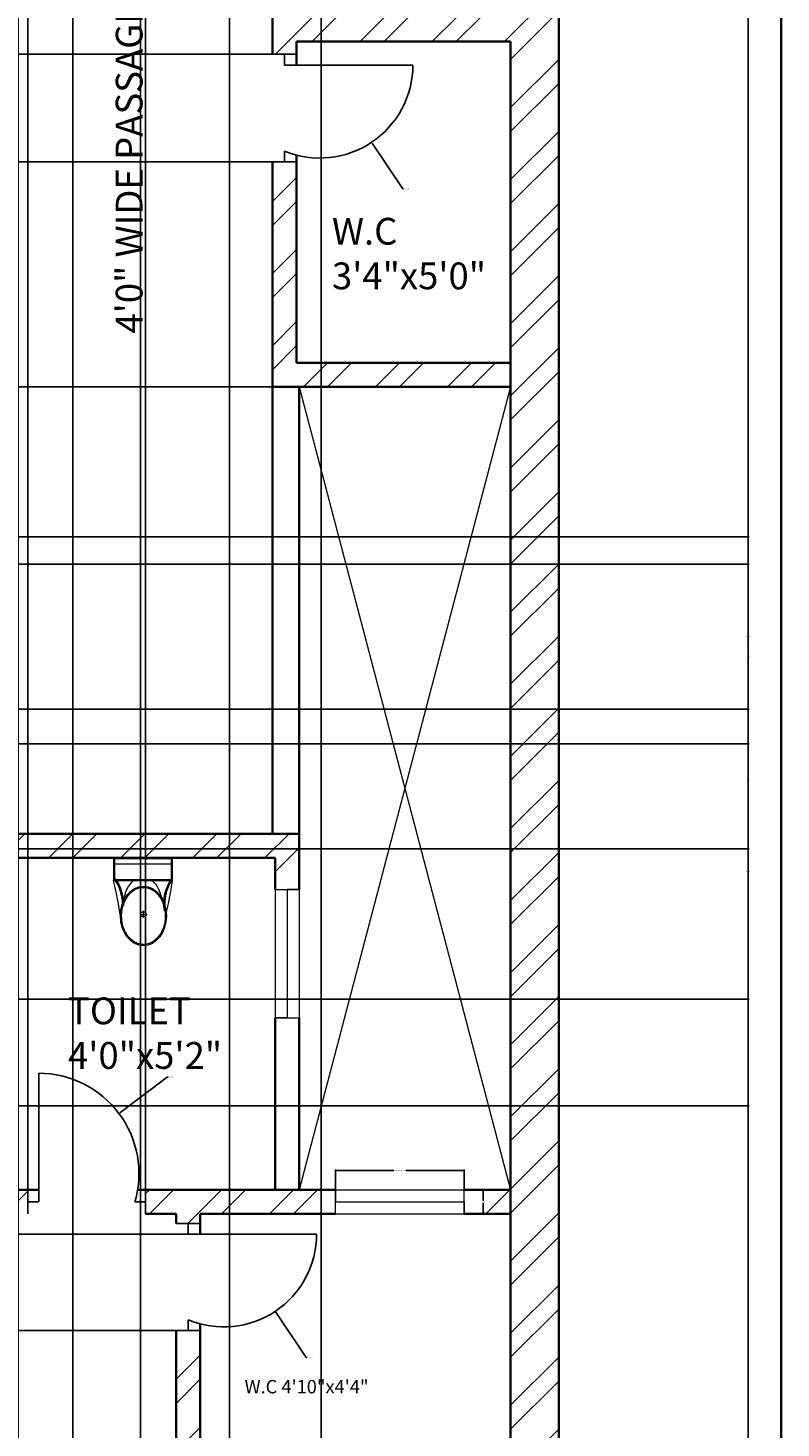
# Model space of a CAD drawing. Units: inches. Extents: x 2529 to 3014, y 1203 to 2262.
# Tile 9 of 13: x 2873 to 3014, y 1746 to 2008. Entities that reach past the tile are written whole.
import ezdxf

# ---------------------------------------------------------------- set-up
doc = ezdxf.new("R2010")
doc.units = ezdxf.units.IN
for name, color, linetype, lineweight in [('A-ANNO-DIMS', 2, 'Continuous', 18), ('A-ANNO-TTLB', 7, 'Continuous', 35), ('A-AREA-IDEN', 7, 'Continuous', 18), ('A-DOOR', 21, 'Continuous', 25), ('A-FLOR-FIXT', 8, 'Continuous', 18), ('A-FLOR-OPEN', 61, 'Continuous', 13), ('A-GLAZ', 191, 'Continuous', 18), ('A-WALL', 7, 'Continuous', 35), ('A-WALL-PATT', 143, 'Continuous', 13)]:
    doc.layers.add(name, color=color, linetype=linetype, lineweight=lineweight)
doc.styles.get("Standard").update_dxf_attribs({"font": 'arial.ttf'})
doc.dimstyles.get("Standard").update_dxf_attribs({"dimtxt": 0.18, "dimasz": 0.18, "dimexe": 0.18, "dimexo": 0.0625, "dimgap": 0.09, "dimtad": 0, "dimtih": 1, "dimtoh": 1, "dimdec": 4, "dimzin": 0, "dimdsep": 46, "dimtxsty": 'Standard', "dimcen": 0.09, "dimadec": 0, "dimazin": 0, "dimtfac": 1, "dimtdec": 4, "dimtofl": 0, "dimtmove": 0, "dimatfit": 3, "dimfxl": 1, "dimtolj": 1, "dimtzin": 0, "dimarcsym": 0})

# ---------------------------------------------------------------- blocks, each defined once
blk = doc.blocks.new('A$C31115884')
for p, q in [((283, 498), (223, 498)), ((258, 466), (258, 523)), ((0, 200), (0, 0)), ((520, 200), (0, 200)), ((10, 190), (10, 10)), ((510, 190), (10, 190)), ((510, 10), (510, 190)), ((520, 0), (520, 200)), ((510, 54), (0, 54)), ((10, 10), (510, 10)), ((0, 0), (520, 0))]:
    blk.add_line(p, q)
blk.add_circle((256, 496), 23.6)
for centre, radius, start, end in [((2778, -205), 2807, 165.4549, 171.7133), ((3237, 905), 2807, 188.2867, 194.5451), ((-295, 403), 365, 324.2091, 9.3499), ((-295, 403), 375, 324.2091, 9.3499), ((139, 406), 293, 315.8436, 2.6563), ((806, 403), 375, 179.2036, 215.7909), ((806, 403), 365, 170.6501, 215.7909), ((384, 406), 293, 190.2774, 224.1564)]:
    blk.add_arc(centre, radius, start, end)
blk.add_ellipse((256, 510), major_axis=(0, -261), ratio=0.772727)
blk.add_open_spline([(256, 259), (263, 259), (270, 260), (288, 262), (299, 265), (320, 273), (330, 278), (350, 291), (360, 299), (378, 316), (386, 326), (402, 347), (409, 358), (421, 383), (427, 395), (436, 422), (440, 436), (445, 465), (447, 480), (448, 509), (448, 524), (445, 553), (443, 568), (436, 596), (432, 610), (422, 636), (416, 649), (402, 672), (395, 683), (379, 703), (370, 712), (351, 728), (341, 735), (321, 746), (310, 751), (289, 757), (278, 759), (256, 761), (245, 761), (223, 757), (212, 754), (191, 746), (181, 741), (161, 728), (151, 720), (133, 703), (125, 693), (110, 672), (103, 660), (90, 636), (85, 623), (76, 596), (72, 582), (67, 553), (66, 538), (64, 509), (65, 494), (68, 465), (70, 450), (77, 422), (81, 408), (91, 382), (97, 370), (111, 346), (118, 335), (135, 316), (144, 307), (162, 291), (172, 284), (193, 273), (203, 269), (225, 262), (236, 260), (250, 259), (253, 259), (256, 259)], degree=3, knots=[0, 0, 0, 0, 0.110105, 0.110105, 0.285049, 0.285049, 0.459994, 0.459994, 0.634938, 0.634938, 0.809882, 0.809882, 0.984827, 0.984827, 1.159771, 1.159771, 1.334715, 1.334715, 1.50966, 1.50966, 1.684604, 1.684604, 1.859549, 1.859549, 2.034493, 2.034493, 2.209437, 2.209437, 2.384382, 2.384382, 2.559326, 2.559326, 2.73427, 2.73427, 2.909215, 2.909215, 3.084159, 3.084159, 3.259103, 3.259103, 3.434048, 3.434048, 3.608992, 3.608992, 3.783936, 3.783936, 3.958881, 3.958881, 4.133825, 4.133825, 4.30877, 4.30877, 4.483714, 4.483714, 4.658658, 4.658658, 4.833603, 4.833603, 5.008547, 5.008547, 5.183491, 5.183491, 5.358436, 5.358436, 5.53338, 5.53338, 5.708324, 5.708324, 5.883269, 5.883269, 6.058213, 6.058213, 6.233158, 6.233158, 6.283185, 6.283185, 6.283185, 6.283185])
blk = doc.blocks.new('WIN-24x4-5')
for p, q in [((0, 24), (4.5, 24)), ((0, 24), (0, 0)), ((4.5, 24), (2.25, 24)), ((2.25, 24), (2.25, 0)), ((4.5, 24), (4.5, 0)), ((2.25, 0), (0, 0)), ((0, 0), (4.5, 0))]:
    blk.add_line(p, q)
blk = doc.blocks.new('*D12')
at = {"layer": 'A-ANNO-DIMS', "color": 0, "lineweight": -2, "transparency": 16777216}
for p, q in [((2930.37, 1791.07), (2930.37, 1794.78)), ((2930.55, 1794.6), (2941.25, 1794.6)), ((2954.19, 1794.6), (2943.49, 1794.6)), ((2954.37, 1791.07), (2954.37, 1794.78))]:
    blk.add_line(p, q, dxfattribs=at)
at = {"layer": 'A-ANNO-DIMS', "color": 0, "transparency": 16777216}
for points in [[(2930.55, 1794.63), (2930.55, 1794.57), (2930.37, 1794.6)], [(2954.19, 1794.63), (2954.19, 1794.57), (2954.37, 1794.6)]]:
    blk.add_solid(points, dxfattribs=at)
at = {"layer": 'Defpoints', "color": 0, "transparency": 16777216}
for p in [(2930.37, 1794.6), (2930.37, 1791), (2954.37, 1791)]:
    blk.add_point(p, dxfattribs=at)
at = {"layer": 'A-ANNO-DIMS', "color": 0, "transparency": 16777216, "insert": (2942.37, 1794.6), "char_height": 0.18, "attachment_point": 5}
blk.add_mtext('\\A1;WINDOW 24 TYP.', dxfattribs=at)
blk = doc.blocks.new('*D13')
at = {"layer": 'A-ANNO-DIMS', "color": 0, "lineweight": -2, "transparency": 16777216}
for p, q in [((2954.43, 1791), (2958.15, 1791)), ((2957.97, 1790.82), (2957.97, 1788.93)), ((2957.97, 1786.68), (2957.97, 1788.57)), ((2954.43, 1786.5), (2958.15, 1786.5))]:
    blk.add_line(p, q, dxfattribs=at)
at = {"layer": 'A-ANNO-DIMS', "color": 0, "transparency": 16777216}
for points in [[(2957.94, 1790.82), (2958, 1790.82), (2957.97, 1791)], [(2957.94, 1786.68), (2958, 1786.68), (2957.97, 1786.5)]]:
    blk.add_solid(points, dxfattribs=at)
at = {"layer": 'Defpoints', "color": 0, "transparency": 16777216}
for p in [(2954.37, 1791), (2957.97, 1791), (2954.37, 1786.5)]:
    blk.add_point(p, dxfattribs=at)
at = {"layer": 'A-ANNO-DIMS', "color": 0, "transparency": 16777216, "insert": (2957.97, 1788.75), "char_height": 0.18, "attachment_point": 5}
blk.add_mtext('\\A1;5 TYP.', dxfattribs=at)
blk = doc.blocks.new('*D17')
at = {"layer": 'A-ANNO-DIMS', "color": 0, "lineweight": -2, "transparency": 16777216}
for p, q in [((2972.12, 2207.5), (3007.66, 2207.5)), ((3007.48, 2207.32), (3007.48, 1890.69)), ((3007.48, 1573.68), (3007.48, 1890.32)), ((2972.12, 1573.5), (3007.66, 1573.5))]:
    blk.add_line(p, q, dxfattribs=at)
at = {"layer": 'A-ANNO-DIMS', "color": 0, "transparency": 16777216}
for points in [[(3007.45, 2207.32), (3007.51, 2207.32), (3007.48, 2207.5)], [(3007.45, 1573.68), (3007.51, 1573.68), (3007.48, 1573.5)]]:
    blk.add_solid(points, dxfattribs=at)
at = {"layer": 'Defpoints', "color": 0, "transparency": 16777216}
for p in [(2972.06, 2207.5), (3007.48, 2207.5), (2972.06, 1573.5)]:
    blk.add_point(p, dxfattribs=at)
at = {"layer": 'A-ANNO-DIMS', "color": 0, "transparency": 16777216, "insert": (3007.48, 1890.5), "char_height": 0.18, "attachment_point": 5}
blk.add_mtext('\\A1;634', dxfattribs=at)
blk = doc.blocks.new('*D39')
at = {"layer": 'A-ANNO-DIMS', "color": 0, "lineweight": -2, "transparency": 16777216}
for p, q in [((2848.27, 1734.07), (2848.27, 2243.11)), ((2848.45, 2242.93), (2864.3, 2242.93)), ((2881.08, 2242.93), (2865.23, 2242.93)), ((2881.26, 1734.07), (2881.26, 2243.11))]:
    blk.add_line(p, q, dxfattribs=at)
at = {"layer": 'A-ANNO-DIMS', "color": 0, "transparency": 16777216}
for points in [[(2848.45, 2242.96), (2848.45, 2242.9), (2848.27, 2242.93)], [(2881.08, 2242.96), (2881.08, 2242.9), (2881.26, 2242.93)]]:
    blk.add_solid(points, dxfattribs=at)
at = {"layer": 'Defpoints', "color": 0, "transparency": 16777216}
for p in [(2881.26, 2242.93), (2848.27, 1734), (2881.26, 1734)]:
    blk.add_point(p, dxfattribs=at)
at = {"layer": 'A-ANNO-DIMS', "color": 0, "transparency": 16777216, "insert": (2864.76, 2242.93), "char_height": 0.18, "attachment_point": 5}
blk.add_mtext('\\A1;32.994', dxfattribs=at)
blk = doc.blocks.new('*D57')
at = {"layer": 'A-ANNO-DIMS', "color": 0, "lineweight": -2, "transparency": 16777216}
for p, q in [((2871.06, 2198.44), (2871.06, 1483.77)), ((2893.92, 2198.44), (2893.92, 1483.77)), ((2871.24, 1483.95), (2882.02, 1483.95)), ((2893.74, 1483.95), (2882.95, 1483.95))]:
    blk.add_line(p, q, dxfattribs=at)
at = {"layer": 'A-ANNO-DIMS', "color": 0, "transparency": 16777216}
for points in [[(2871.24, 1483.98), (2871.24, 1483.92), (2871.06, 1483.95)], [(2893.74, 1483.98), (2893.74, 1483.92), (2893.92, 1483.95)]]:
    blk.add_solid(points, dxfattribs=at)
at = {"layer": 'Defpoints', "color": 0, "transparency": 16777216}
for p in [(2871.06, 2198.5), (2893.92, 2198.5), (2893.92, 1483.95)]:
    blk.add_point(p, dxfattribs=at)
at = {"layer": 'A-ANNO-DIMS', "color": 0, "transparency": 16777216, "insert": (2882.49, 1483.95), "char_height": 0.18, "attachment_point": 5}
blk.add_mtext('\\A1;22.866', dxfattribs=at)
blk = doc.blocks.new('*D60')
at = {"layer": 'A-ANNO-DIMS', "color": 0, "lineweight": -2, "transparency": 16777216}
for p, q in [((2918.49, 2003.13), (2541.45, 2003.13)), ((2541.63, 2002.95), (2541.63, 1993.28)), ((2541.63, 1983.24), (2541.63, 1992.91)), ((2918.49, 1983.06), (2541.45, 1983.06))]:
    blk.add_line(p, q, dxfattribs=at)
at = {"layer": 'A-ANNO-DIMS', "color": 0, "transparency": 16777216}
for points in [[(2541.6, 2002.95), (2541.66, 2002.95), (2541.63, 2003.13)], [(2541.6, 1983.24), (2541.66, 1983.24), (2541.63, 1983.06)]]:
    blk.add_solid(points, dxfattribs=at)
at = {"layer": 'Defpoints', "color": 0, "transparency": 16777216}
for p in [(2918.56, 2003.13), (2541.63, 1983.06), (2918.56, 1983.06)]:
    blk.add_point(p, dxfattribs=at)
at = {"layer": 'A-ANNO-DIMS', "color": 0, "transparency": 16777216, "insert": (2541.63, 1993.1), "char_height": 0.18, "attachment_point": 5}
blk.add_mtext('\\A1;20.077', dxfattribs=at)
blk = doc.blocks.new('*D61')
at = {"layer": 'A-ANNO-DIMS', "color": 0, "lineweight": -2, "transparency": 16777216}
for p, q in [((2918.49, 1983.06), (2541.45, 1983.06)), ((2541.63, 1982.88), (2541.63, 1962.21)), ((2541.63, 1941.18), (2541.63, 1961.85)), ((2918.49, 1941), (2541.45, 1941))]:
    blk.add_line(p, q, dxfattribs=at)
at = {"layer": 'A-ANNO-DIMS', "color": 0, "transparency": 16777216}
for points in [[(2541.6, 1982.88), (2541.66, 1982.88), (2541.63, 1983.06)], [(2541.6, 1941.18), (2541.66, 1941.18), (2541.63, 1941)]]:
    blk.add_solid(points, dxfattribs=at)
at = {"layer": 'Defpoints', "color": 0, "transparency": 16777216}
for p in [(2918.56, 1983.06), (2541.63, 1941), (2918.56, 1941)]:
    blk.add_point(p, dxfattribs=at)
at = {"layer": 'A-ANNO-DIMS', "color": 0, "transparency": 16777216, "insert": (2541.63, 1962.03), "char_height": 0.18, "attachment_point": 5}
blk.add_mtext('\\A1;42.05', dxfattribs=at)
blk = doc.blocks.new('*D62')
at = {"layer": 'A-ANNO-DIMS', "color": 0, "lineweight": -2, "transparency": 16777216}
for p, q in [((2904.99, 1782.69), (2541.45, 1782.69)), ((2541.63, 1782.51), (2541.63, 1773.88)), ((2541.63, 1764.89), (2541.63, 1773.52)), ((2904.99, 1764.71), (2541.45, 1764.71))]:
    blk.add_line(p, q, dxfattribs=at)
at = {"layer": 'A-ANNO-DIMS', "color": 0, "transparency": 16777216}
for points in [[(2541.6, 1782.51), (2541.66, 1782.51), (2541.63, 1782.69)], [(2541.6, 1764.89), (2541.66, 1764.89), (2541.63, 1764.71)]]:
    blk.add_solid(points, dxfattribs=at)
at = {"layer": 'Defpoints', "color": 0, "transparency": 16777216}
for p in [(2905.06, 1782.69), (2541.63, 1764.71), (2905.06, 1764.71)]:
    blk.add_point(p, dxfattribs=at)
at = {"layer": 'A-ANNO-DIMS', "color": 0, "transparency": 16777216, "insert": (2541.63, 1773.7), "char_height": 0.18, "attachment_point": 5}
blk.add_mtext('\\A1;17.983', dxfattribs=at)
blk = doc.blocks.new('*D63')
at = {"layer": 'A-ANNO-DIMS', "color": 0, "lineweight": -2, "transparency": 16777216}
for p, q in [((2737.62, 1907.87), (3007.66, 1907.87)), ((3007.48, 1907.69), (3007.48, 1894.52)), ((3007.48, 1880.99), (3007.48, 1894.16)), ((2737.62, 1880.81), (3007.66, 1880.81))]:
    blk.add_line(p, q, dxfattribs=at)
at = {"layer": 'A-ANNO-DIMS', "color": 0, "transparency": 16777216}
for points in [[(3007.45, 1907.69), (3007.51, 1907.69), (3007.48, 1907.87)], [(3007.45, 1880.99), (3007.51, 1880.99), (3007.48, 1880.81)]]:
    blk.add_solid(points, dxfattribs=at)
at = {"layer": 'Defpoints', "color": 0, "transparency": 16777216}
for p in [(2737.56, 1907.87), (3007.48, 1907.87), (2737.56, 1880.81)]:
    blk.add_point(p, dxfattribs=at)
at = {"layer": 'A-ANNO-DIMS', "color": 0, "transparency": 16777216, "insert": (3007.48, 1894.34), "char_height": 0.18, "attachment_point": 5}
blk.add_mtext('\\A1;27.057', dxfattribs=at)
blk = doc.blocks.new('*D64')
at = {"layer": 'A-ANNO-DIMS', "color": 0, "lineweight": -2, "transparency": 16777216}
for p, q in [((2872.87, 1791.07), (2872.87, 2243.11)), ((2873.05, 2242.93), (2883.47, 2242.93)), ((2894.68, 2242.93), (2884.26, 2242.93)), ((2894.86, 1791.07), (2894.86, 2243.11))]:
    blk.add_line(p, q, dxfattribs=at)
at = {"layer": 'A-ANNO-DIMS', "color": 0, "transparency": 16777216}
for points in [[(2873.05, 2242.96), (2873.05, 2242.9), (2872.87, 2242.93)], [(2894.68, 2242.96), (2894.68, 2242.9), (2894.86, 2242.93)]]:
    blk.add_solid(points, dxfattribs=at)
at = {"layer": 'Defpoints', "color": 0, "transparency": 16777216}
for p in [(2894.86, 2242.93), (2872.87, 1791), (2894.86, 1791)]:
    blk.add_point(p, dxfattribs=at)
at = {"layer": 'A-ANNO-DIMS', "color": 0, "transparency": 16777216, "insert": (2883.87, 2242.93), "char_height": 0.18, "attachment_point": 5}
blk.add_mtext('\\A1;21.99', dxfattribs=at)
blk = doc.blocks.new('*D67')
at = {"layer": 'A-ANNO-DIMS', "color": 0, "lineweight": -2, "transparency": 16777216}
for p, q in [((2678.12, 1913), (3007.66, 1913)), ((3007.48, 1912.82), (3007.48, 1893.83)), ((3007.48, 1874.48), (3007.48, 1893.47)), ((2678.12, 1874.3), (3007.66, 1874.3))]:
    blk.add_line(p, q, dxfattribs=at)
at = {"layer": 'A-ANNO-DIMS', "color": 0, "transparency": 16777216}
for points in [[(3007.45, 1912.82), (3007.51, 1912.82), (3007.48, 1913)], [(3007.45, 1874.48), (3007.51, 1874.48), (3007.48, 1874.3)]]:
    blk.add_solid(points, dxfattribs=at)
at = {"layer": 'Defpoints', "color": 0, "transparency": 16777216}
for p in [(2678.06, 1913), (3007.48, 1913), (2678.06, 1874.3)]:
    blk.add_point(p, dxfattribs=at)
at = {"layer": 'A-ANNO-DIMS', "color": 0, "transparency": 16777216, "insert": (3007.48, 1893.65), "char_height": 0.18, "attachment_point": 5}
blk.add_mtext('\\A1;38.7', dxfattribs=at)
blk = doc.blocks.new('*D68')
at = {"layer": 'A-ANNO-DIMS', "color": 0, "lineweight": -2, "transparency": 16777216}
for p, q in [((2622.12, 1874.3), (3007.66, 1874.3)), ((3007.48, 1874.12), (3007.48, 1850.62)), ((3007.48, 1826.75), (3007.48, 1850.25)), ((2622.12, 1826.57), (3007.66, 1826.57))]:
    blk.add_line(p, q, dxfattribs=at)
at = {"layer": 'A-ANNO-DIMS', "color": 0, "transparency": 16777216}
for points in [[(3007.45, 1874.12), (3007.51, 1874.12), (3007.48, 1874.3)], [(3007.45, 1826.75), (3007.51, 1826.75), (3007.48, 1826.57)]]:
    blk.add_solid(points, dxfattribs=at)
at = {"layer": 'Defpoints', "color": 0, "transparency": 16777216}
for p in [(2622.06, 1874.3), (3007.48, 1874.3), (2622.06, 1826.57)]:
    blk.add_point(p, dxfattribs=at)
at = {"layer": 'A-ANNO-DIMS', "color": 0, "transparency": 16777216, "insert": (3007.48, 1850.43), "char_height": 0.18, "attachment_point": 5}
blk.add_mtext('\\A1;47.735', dxfattribs=at)
blk = doc.blocks.new('*D69')
at = {"layer": 'A-ANNO-DIMS', "color": 0, "lineweight": -2, "transparency": 16777216}
for p, q in [((2737.62, 1854.67), (3007.66, 1854.67)), ((3007.48, 1854.49), (3007.48, 1830.85)), ((3007.48, 1806.85), (3007.48, 1830.49)), ((2737.62, 1806.67), (3007.66, 1806.67))]:
    blk.add_line(p, q, dxfattribs=at)
at = {"layer": 'A-ANNO-DIMS', "color": 0, "transparency": 16777216}
for points in [[(3007.45, 1854.49), (3007.51, 1854.49), (3007.48, 1854.67)], [(3007.45, 1806.85), (3007.51, 1806.85), (3007.48, 1806.67)]]:
    blk.add_solid(points, dxfattribs=at)
at = {"layer": 'Defpoints', "color": 0, "transparency": 16777216}
for p in [(2737.56, 1854.67), (3007.48, 1854.67), (2737.56, 1806.67)]:
    blk.add_point(p, dxfattribs=at)
at = {"layer": 'A-ANNO-DIMS', "color": 0, "transparency": 16777216, "insert": (3007.48, 1830.67), "char_height": 0.18, "attachment_point": 5}
blk.add_mtext('\\A1;48', dxfattribs=at)
blk = doc.blocks.new('*D70')
at = {"layer": 'A-ANNO-DIMS', "color": 0, "lineweight": -2, "transparency": 16777216}
for p, q in [((2737.62, 1880.81), (3007.66, 1880.81)), ((3007.48, 1880.63), (3007.48, 1867.92)), ((3007.48, 1854.85), (3007.48, 1867.56)), ((2737.62, 1854.67), (3007.66, 1854.67))]:
    blk.add_line(p, q, dxfattribs=at)
at = {"layer": 'A-ANNO-DIMS', "color": 0, "transparency": 16777216}
for points in [[(3007.45, 1880.63), (3007.51, 1880.63), (3007.48, 1880.81)], [(3007.45, 1854.85), (3007.51, 1854.85), (3007.48, 1854.67)]]:
    blk.add_solid(points, dxfattribs=at)
at = {"layer": 'Defpoints', "color": 0, "transparency": 16777216}
for p in [(2737.56, 1880.81), (3007.48, 1880.81), (2737.56, 1854.67)]:
    blk.add_point(p, dxfattribs=at)
at = {"layer": 'A-ANNO-DIMS', "color": 0, "transparency": 16777216, "insert": (3007.48, 1867.74), "char_height": 0.18, "attachment_point": 5}
blk.add_mtext('\\A1;26.14', dxfattribs=at)
blk = doc.blocks.new('*D75')
at = {"layer": 'A-ANNO-DIMS', "color": 0, "lineweight": -2, "transparency": 16777216}
for p, q in [((2893.92, 2187.06), (2893.92, 1483.77)), ((2910.52, 2189.17), (2910.52, 1483.77)), ((2894.1, 1483.95), (2901.91, 1483.95)), ((2910.34, 1483.95), (2902.54, 1483.95))]:
    blk.add_line(p, q, dxfattribs=at)
at = {"layer": 'A-ANNO-DIMS', "color": 0, "transparency": 16777216}
for points in [[(2894.1, 1483.98), (2894.1, 1483.92), (2893.92, 1483.95)], [(2910.34, 1483.98), (2910.34, 1483.92), (2910.52, 1483.95)]]:
    blk.add_solid(points, dxfattribs=at)
at = {"layer": 'Defpoints', "color": 0, "transparency": 16777216}
for p in [(2893.92, 2187.12), (2910.52, 2189.24), (2910.52, 1483.95)]:
    blk.add_point(p, dxfattribs=at)
at = {"layer": 'A-ANNO-DIMS', "color": 0, "transparency": 16777216, "insert": (2902.22, 1483.95), "char_height": 0.18, "attachment_point": 5}
blk.add_mtext('\\A1;16.6', dxfattribs=at)
blk = doc.blocks.new('*D76')
at = {"layer": 'A-ANNO-DIMS', "color": 0, "lineweight": -2, "transparency": 16777216}
for p, q in [((2910.52, 2189.17), (2910.52, 1483.77)), ((2927.64, 2189.17), (2927.64, 1483.77)), ((2910.7, 1483.95), (2918.63, 1483.95)), ((2927.46, 1483.95), (2919.54, 1483.95))]:
    blk.add_line(p, q, dxfattribs=at)
at = {"layer": 'A-ANNO-DIMS', "color": 0, "transparency": 16777216}
for points in [[(2910.7, 1483.98), (2910.7, 1483.92), (2910.52, 1483.95)], [(2927.46, 1483.98), (2927.46, 1483.92), (2927.64, 1483.95)]]:
    blk.add_solid(points, dxfattribs=at)
at = {"layer": 'Defpoints', "color": 0, "transparency": 16777216}
for p in [(2910.52, 2189.24), (2927.64, 2189.24), (2927.64, 1483.95)]:
    blk.add_point(p, dxfattribs=at)
at = {"layer": 'A-ANNO-DIMS', "color": 0, "transparency": 16777216, "insert": (2919.08, 1483.95), "char_height": 0.18, "attachment_point": 5}
blk.add_mtext('\\A1;17.123', dxfattribs=at)
blk = doc.blocks.new('*D88')
at = {"layer": 'A-ANNO-DIMS', "color": 0, "lineweight": -2, "transparency": 16777216}
for p, q in [((2898.87, 1812), (2890.02, 1805.36)), ((2899.05, 1812), (2898.87, 1812)), ((2874.78, 1794.01), (2874.96, 1794.01)), ((2874.87, 1793.92), (2874.87, 1794.1))]:
    blk.add_line(p, q, dxfattribs=at)
at = {"layer": 'A-ANNO-DIMS', "color": 0, "transparency": 16777216}
blk.add_solid([(2890, 1805.38), (2890.03, 1805.34), (2889.87, 1805.25)], dxfattribs=at)
at = {"layer": 'Defpoints', "color": 0, "transparency": 16777216}
for p in [(2889.87, 1805.25), (2874.87, 1794.01)]:
    blk.add_point(p, dxfattribs=at)
at = {"layer": 'A-ANNO-DIMS', "color": 0, "transparency": 16777216, "insert": (2899.6, 1812), "char_height": 0.18, "attachment_point": 5}
blk.add_mtext('\\A1;R18.742', dxfattribs=at)
blk = doc.blocks.new('*D90')
at = {"layer": 'A-ANNO-DIMS', "color": 0, "lineweight": -2, "transparency": 16777216}
for p, q in [((2927.33, 2001.13), (2927.51, 2001.13)), ((2927.42, 2001.04), (2927.42, 2001.22)), ((2942.9, 1978.02), (2937.2, 1986.54)), ((2943.08, 1978.02), (2942.9, 1978.02))]:
    blk.add_line(p, q, dxfattribs=at)
at = {"layer": 'A-ANNO-DIMS', "color": 0, "transparency": 16777216}
blk.add_solid([(2937.22, 1986.56), (2937.17, 1986.52), (2937.1, 1986.69)], dxfattribs=at)
at = {"layer": 'Defpoints', "color": 0, "transparency": 16777216}
for p in [(2927.42, 2001.13), (2937.1, 1986.69)]:
    blk.add_point(p, dxfattribs=at)
at = {"layer": 'A-ANNO-DIMS', "color": 0, "transparency": 16777216, "insert": (2943.63, 1978.02), "char_height": 0.18, "attachment_point": 5}
blk.add_mtext('\\A1;R17.385', dxfattribs=at)
blk = doc.blocks.new('*D91')
at = {"layer": 'A-ANNO-DIMS', "color": 0, "lineweight": -2, "transparency": 16777216}
for p, q in [((2909.39, 1782.69), (2909.57, 1782.69)), ((2909.48, 1782.6), (2909.48, 1782.78)), ((2924.85, 1759.62), (2919.18, 1768.13)), ((2925.03, 1759.62), (2924.85, 1759.62))]:
    blk.add_line(p, q, dxfattribs=at)
at = {"layer": 'A-ANNO-DIMS', "color": 0, "transparency": 16777216}
blk.add_solid([(2919.21, 1768.14), (2919.16, 1768.11), (2919.08, 1768.28)], dxfattribs=at)
at = {"layer": 'Defpoints', "color": 0, "transparency": 16777216}
for p in [(2909.48, 1782.69), (2919.08, 1768.28)]:
    blk.add_point(p, dxfattribs=at)
at = {"layer": 'A-ANNO-DIMS', "color": 0, "transparency": 16777216, "insert": (2925.57, 1759.62), "char_height": 0.18, "attachment_point": 5}
blk.add_mtext('\\A1;R17.322', dxfattribs=at)

msp = doc.modelspace()

# ---------------------------------------------------------------- hatches: boundary and pattern name
at = {"layer": 'A-WALL-PATT'}
h = msp.add_hatch(dxfattribs=at)
h.set_pattern_fill('ANSI32', color=256)
h.paths.add_polyline_path([(2686.5554, 2106.5032), (2622.0554, 2106.5032), (2622.0554, 2109.2964), (2617.4223, 2109.2964), (2613.0554, 2109.2964), (2613.0554, 2106.5032), (2577.0554, 2106.5032), (2577.0554, 2092.6918), (2586.0554, 2092.6918), (2586.0554, 2102.0032), (2682.0554, 2102.0032), (2682.0554, 2099.9833), (2686.5554, 2099.9833), (2686.5554, 2102.0032)])
h.paths.add_polyline_path([(2695.2249, 2054.0032), (2686.5554, 2054.0032), (2686.5554, 2080.2316), (2684.3054, 2080.2316), (2682.0554, 2080.2316), (2682.0554, 2054.0032), (2586.0554, 2054.0032), (2586.0554, 2068.6918), (2577.0554, 2068.6918), (2577.0554, 2019.1229), (2586.0554, 2019.1229), (2586.0554, 2049.5032), (2695.2249, 2049.5032)])
h.paths.add_polyline_path([(2737.5554, 2049.5032), (2866.5554, 2049.5032), (2866.5554, 2045.0233), (2871.0554, 2045.0233), (2871.0554, 2049.5032), (2871.0554, 2172.5032), (2866.5554, 2172.5032), (2829.1265, 2172.5032), (2829.1265, 2168.0032), (2866.5554, 2168.0032), (2866.5554, 2054.0032), (2737.5554, 2054.0032), (2737.5554, 2056.4892), (2735.3054, 2056.4892), (2733.0554, 2056.4892), (2733.0554, 2049.5032), (2733.0554, 1917.5032), (2733.0554, 1913.0032), (2871.0554, 1913.0032), (2871.0554, 1924.9149), (2868.8054, 1924.9149), (2866.5554, 1924.9149), (2866.5554, 1917.5032), (2737.5554, 1917.5032)], flags=17)
h.paths.add_polyline_path([(2972.0554, 2207.5032), (2613.0554, 2207.5032), (2613.0554, 2205.5032), (2613.0554, 2188.9366), (2622.0554, 2188.9366), (2622.0554, 2198.5032), (2733.0554, 2198.5032), (2733.0554, 2084.8053), (2735.3054, 2084.8053), (2737.5554, 2084.8053), (2737.5554, 2168.0032), (2769.1265, 2168.0032), (2769.1265, 2170.2532), (2769.1265, 2172.5032), (2737.5554, 2172.5032), (2737.5554, 2198.5032), (2963.0554, 2198.5032), (2963.0554, 2093.5032), (2912.0586, 2093.5032), (2912.0586, 2089.0032), (2918.5554, 2089.0032), (2918.5554, 2031.8749), (2923.0554, 2031.8749), (2923.0554, 2089.0032), (2963.0554, 2089.0032), (2963.0554, 2010.0032), (2923.0554, 2010.0032), (2923.0554, 2011.9417), (2918.5554, 2011.9417), (2918.5554, 2003.1338), (2923.0554, 2003.1338), (2923.0554, 2005.5032), (2963.0554, 2005.5032), (2963.0554, 1917.5032), (2963.0554, 1691.0776), (2972.0554, 1691.0776), (2972.0554, 1917.5032)])
h.paths.add_polyline_path([(2963.0554, 1945.5032), (2923.0554, 1945.5032), (2923.0554, 1983.0571), (2920.8054, 1983.0571), (2918.5554, 1983.0571), (2918.5554, 1941.0032), (2963.0554, 1941.0032)], flags=17)
h.paths.add_polyline_path([(2930.3679, 1788.7532), (2930.3679, 1791.0032), (2894.8637, 1791.0032), (2894.8637, 1786.5032), (2900.5554, 1786.5032), (2900.5554, 1784.6931), (2905.0554, 1784.6931), (2905.0554, 1786.5032), (2930.3679, 1786.5032)], flags=17)
h.paths.add_polyline_path([(2963.0554, 1791.0032), (2954.3679, 1791.0032), (2954.3679, 1786.5032), (2963.0554, 1786.5032)], flags=17)
h.paths.add_polyline_path([(2871.0554, 1853.0032), (2919.0554, 1853.0032), (2919.0554, 1847.0972), (2923.5554, 1847.0972), (2923.5554, 1853.0032), (2923.5554, 1857.5032), (2871.0554, 1857.5032), (2871.0554, 1871.7024), (2866.5554, 1871.7024), (2866.5554, 1791.0032), (2737.5554, 1791.0032), (2737.5554, 1806.6712), (2735.3054, 1806.6712), (2733.0554, 1806.6712), (2733.0554, 1791.0032), (2733.0554, 1786.5032), (2733.0554, 1780.6235), (2737.5554, 1780.6235), (2737.5554, 1786.5032), (2872.8745, 1786.5032), (2872.8745, 1788.7532), (2872.8745, 1791.0032), (2871.0554, 1791.0032)], flags=17)
h.paths.add_polyline_path([(2844.0554, 1734.0032), (2848.2652, 1734.0032), (2848.2652, 1738.5032), (2800.0167, 1738.5032), (2800.0167, 1734.0032), (2839.5554, 1734.0032), (2839.5554, 1582.5032), (2792.3334, 1582.5032), (2792.3334, 1573.5032), (2871.4433, 1573.5032), (2871.4433, 1578.0032), (2871.4433, 1582.5032), (2844.0554, 1582.5032)])
h.paths.add_polyline_path([(2972.0554, 1631.0776), (2963.0554, 1631.0776), (2963.0554, 1582.5032), (2931.4433, 1582.5032), (2931.4433, 1573.5032), (2972.0554, 1573.5032)])
h.paths.add_polyline_path([(2756.3334, 1582.5032), (2737.5554, 1582.5032), (2737.5554, 1734.0032), (2744.3201, 1734.0032), (2744.3201, 1738.5032), (2737.5554, 1738.5032), (2737.5554, 1746.0094), (2733.0554, 1746.0094), (2733.0554, 1738.5032), (2733.0554, 1612.5032), (2728.2475, 1612.5032), (2728.2475, 1603.5032), (2733.0554, 1603.5032), (2733.0554, 1582.5032), (2733.0554, 1573.5032), (2756.3334, 1573.5032), (2756.3334, 1578.0032)])
h.paths.add_polyline_path([(2695.7662, 1612.5032), (2658.4771, 1612.5032), (2658.4771, 1603.5032), (2695.7662, 1603.5032), (2695.7662, 1608.0032)])
h.paths.add_polyline_path([(2586.0554, 1686.9483), (2577.0554, 1686.9483), (2577.0554, 1603.5032), (2598.4771, 1603.5032), (2598.4771, 1608.0032), (2598.4771, 1612.5032), (2586.0554, 1612.5032)])
h.paths.add_polyline_path([(2683.2727, 1791.0032), (2586.0554, 1791.0032), (2586.0554, 1815.6736), (2581.5554, 1815.6736), (2577.0554, 1815.6736), (2577.0554, 1746.9483), (2586.0554, 1746.9483), (2586.0554, 1786.5032), (2683.2727, 1786.5032)])
h.paths.add_polyline_path([(2586.0554, 1959.1229), (2577.0554, 1959.1229), (2577.0554, 1875.6736), (2586.0554, 1875.6736), (2586.0554, 1913.0032), (2683.2727, 1913.0032), (2683.2727, 1917.5032), (2586.0554, 1917.5032)])
h = msp.add_hatch(dxfattribs=at)
h.set_pattern_fill('ANSI32', color=256)
h.paths.add_polyline_path([(2737.5554, 1786.5032), (2872.8745, 1786.5032), (2872.8745, 1788.7532), (2872.8745, 1791.0032), (2871.0554, 1791.0032), (2871.0554, 1853.0032), (2919.0554, 1853.0032), (2919.0554, 1847.0972), (2923.5554, 1847.0972), (2923.5554, 1853.0032), (2923.5554, 1857.5032), (2871.0554, 1857.5032), (2871.0554, 1871.7024), (2866.5554, 1871.7024), (2866.5554, 1791.0032), (2737.5554, 1791.0032), (2737.5554, 1806.6712), (2735.3054, 1806.6712), (2733.0554, 1806.6712), (2733.0554, 1791.0032), (2730.085, 1791.0032), (2730.085, 1786.5032), (2733.0554, 1786.5032), (2733.0554, 1780.6235), (2737.5554, 1780.6235)])
h.paths.add_polyline_path([(2737.5554, 1880.8133), (2735.3054, 1880.8133), (2733.0554, 1880.8133), (2733.0554, 1854.6712), (2737.5554, 1854.6712)])
h.paths.add_polyline_path([(2695.1228, 1915.2532), (2695.1228, 1917.5032), (2586.0554, 1917.5032), (2586.0554, 1959.1229), (2577.0554, 1959.1229), (2577.0554, 1875.6736), (2586.0554, 1875.6736), (2586.0554, 1913.0032), (2695.1228, 1913.0032)])
h = msp.add_hatch(dxfattribs=at)
h.set_pattern_fill('ANSI32', color=256)
h.paths.add_polyline_path([(2696.9325, 1791.0032), (2586.0554, 1791.0032), (2586.0554, 1815.6736), (2581.5554, 1815.6736), (2577.0554, 1815.6736), (2577.0554, 1746.9483), (2586.0554, 1746.9483), (2586.0554, 1786.5032), (2696.9325, 1786.5032)])
h.paths.add_polyline_path([(2872.8745, 1791.0032), (2871.0554, 1791.0032), (2871.0554, 1853.0032), (2919.0554, 1853.0032), (2919.0554, 1847.0972), (2923.5554, 1847.0972), (2923.5554, 1853.0032), (2923.5554, 1857.5032), (2871.0554, 1857.5032), (2871.0554, 1871.7024), (2866.5554, 1871.7024), (2866.5554, 1791.0032), (2737.5554, 1791.0032), (2737.5554, 1806.6712), (2735.3054, 1806.6712), (2733.0554, 1806.6712), (2733.0554, 1791.0032), (2730.085, 1791.0032), (2730.085, 1786.5032), (2733.0554, 1786.5032), (2733.0554, 1780.6235), (2737.5554, 1780.6235), (2737.5554, 1786.5032), (2872.8745, 1786.5032), (2872.8745, 1788.7532)])
h = msp.add_hatch(dxfattribs=at)
h.set_pattern_fill('ANSI32', color=256)
h.paths.add_polyline_path([(2963.0554, 1738.5032), (2905.0554, 1738.5032), (2905.0554, 1764.7097), (2900.5554, 1764.7097), (2900.5554, 1738.5032), (2881.259, 1738.5032), (2881.259, 1734.0032), (2963.0554, 1734.0032)])

# ---------------------------------------------------------------- linework, layer by layer
at = {"layer": 'A-ANNO-TTLB'}
msp.add_lwpolyline([(2528.6765, 2261.8165), (3013.6003, 2261.8165), (3013.6003, 1455.1523), (2528.6765, 1455.1523)], close=True, dxfattribs=at)
at = {"layer": 'A-DOOR'}
for p, q in [((2918.5554, 2003.1338), (2923.0554, 2003.1338)), ((2923.0554, 2003.1338), (2920.8054, 2003.1338)), ((2920.8054, 2003.1338), (2920.8054, 2001.1338)), ((2920.8054, 2001.1338), (2944.8054, 2001.1338)), ((2918.5554, 1983.0571), (2923.0554, 1983.0571)), ((2920.8054, 1983.0571), (2920.8054, 1985.0571)), ((2923.0554, 1983.0571), (2920.8054, 1983.0571)), ((2874.8745, 1788.7532), (2874.8745, 1812.7532)), ((2872.8745, 1791.0032), (2872.8745, 1786.5032)), ((2894.8637, 1791.0032), (2894.8637, 1786.5032)), ((2872.8745, 1786.5032), (2872.8745, 1788.7532)), ((2872.8745, 1788.7532), (2874.8745, 1788.7532)), ((2894.8637, 1788.7532), (2892.8637, 1788.7532)), ((2894.8637, 1786.5032), (2894.8637, 1788.7532)), ((2900.5554, 1784.6931), (2905.0554, 1784.6931)), ((2905.0554, 1784.6931), (2902.8054, 1784.6931)), ((2902.8054, 1784.6931), (2902.8054, 1782.6931)), ((2902.8054, 1782.6931), (2926.8054, 1782.6931)), ((2902.8054, 1764.7097), (2902.8054, 1766.7097)), ((2905.0554, 1764.7097), (2900.5554, 1764.7097)), ((2900.5554, 1764.7097), (2902.8054, 1764.7097))]:
    msp.add_line(p, q, dxfattribs=at)
for centre, radius, start, end in [((2927.4208, 2001.1338), 17.3845, 247.633098, 0), ((2874.8745, 1794.0113), 18.7419, 343.706784, 90), ((2909.4831, 1782.6931), 17.3223, 247.325371, 0)]:
    msp.add_arc(centre, radius, start, end, dxfattribs=at)
at = {"layer": 'A-FLOR-OPEN'}
for p, q in [((2963.0554, 1941.0032), (2923.5554, 1791.0032)), ((2923.5554, 1941.0032), (2963.0554, 1791.0032))]:
    msp.add_line(p, q, dxfattribs=at)
at = {"layer": 'A-WALL'}
for p, q in [((2972.0554, 2207.5032), (2972.0554, 1917.5032)), ((2918.5554, 2011.9417), (2918.5554, 2003.1338)), ((2923.0554, 2005.5032), (2963.0554, 2005.5032)), ((2923.0554, 2005.5032), (2923.0554, 2001.1338)), ((2963.0554, 2005.5032), (2963.0554, 1917.5032)), ((2918.5554, 1983.0571), (2918.5554, 1941.0032)), ((2923.0554, 1984.3063), (2923.0554, 1945.5032)), ((2923.0554, 1945.5032), (2963.0554, 1945.5032)), ((2918.5554, 1941.0032), (2963.0554, 1941.0032)), ((2918.5554, 1941.0032), (2918.5554, 1857.5032)), ((2923.5554, 1857.5032), (2923.5554, 1941.0032)), ((2963.0554, 1691.0776), (2963.0554, 1917.5032)), ((2972.0554, 1917.5032), (2972.0554, 1691.0776)), ((2923.5554, 1857.5032), (2871.0554, 1857.5032)), ((2923.5554, 1853.0032), (2923.5554, 1857.5032)), ((2871.0554, 1853.0032), (2919.0554, 1853.0032)), ((2919.0554, 1853.0032), (2919.0554, 1847.0972)), ((2923.5554, 1847.0972), (2923.5554, 1853.0032)), ((2919.0554, 1823.0972), (2919.0554, 1791.0032)), ((2923.5554, 1791.0032), (2923.5554, 1823.0972)), ((2871.0554, 1791.0032), (2874.8745, 1791.0032)), ((2893.3734, 1791.0032), (2930.3679, 1791.0032)), ((2919.0554, 1791.0032), (2923.5554, 1791.0032)), ((2954.3679, 1791.0032), (2963.0554, 1791.0032)), ((2894.8637, 1786.5032), (2900.5554, 1786.5032)), ((2900.5554, 1786.5032), (2900.5554, 1784.6931)), ((2905.0554, 1786.5032), (2930.3679, 1786.5032)), ((2905.0554, 1782.6931), (2905.0554, 1786.5032)), ((2954.3679, 1786.5032), (2963.0554, 1786.5032)), ((2963.0554, 1786.5032), (2963.0554, 1734.5032)), ((2905.0554, 1738.5032), (2905.0554, 1765.9462)), ((2900.5554, 1764.7097), (2900.5554, 1738.5032))]:
    msp.add_line(p, q, dxfattribs=at)

# ---------------------------------------------------------------- block references
at = {"layer": 'A-FLOR-FIXT', "xscale": 0.021283599635143, "yscale": 0.021283599635143, "zscale": 0.021283599635143, "rotation": 180}
msp.add_blockref('A$C31115884', (2899.9039, 1853.0032), dxfattribs=at)
at = {"layer": 'A-GLAZ'}
msp.add_blockref('WIN-24x4-5', (2919.055, 1823.097), dxfattribs=at)
at = {"layer": 'A-GLAZ', "rotation": 90.00000000000335}
msp.add_blockref('WIN-24x4-5', (2954.3681, 1786.5029), dxfattribs=at)

# ---------------------------------------------------------------- texts
at = {"layer": 'A-AREA-IDEN', "insert": (2889.2755, 1950.9524), "char_height": 5, "attachment_point": 1, "rotation": 90}
msp.add_mtext_dynamic_manual_height_columns('4\'0" WIDE PASSAGE', width=108.755322, gutter_width=12.5, heights=[0], dxfattribs=at)
at = {"layer": 'A-AREA-IDEN', "attachment_point": 1}
for s, width, insert, char_height in [('W.C\\P3\'4"x5\'0"', 69.763602, (2929.6789, 1972.5721), 5), ('TOILET\\P4\'0"x5\'2"', 78.14858, (2880.356, 1826.9124), 5), ('W.C 4\'10"x4\'4"', 99.725697, (2913.3488, 1755.4515), 2.5)]:
    msp.add_mtext_dynamic_manual_height_columns(s, width=width, gutter_width=12.5, heights=[0], dxfattribs=dict(at, insert=insert, char_height=char_height))

# ---------------------------------------------------------------- dimensions: what is measured, and where the dimension line sits
at = {"layer": 'A-ANNO-DIMS'}
for base, p1, p2, override, picture, middle in [((2881.259, 2242.9282), (2848.2652, 1734.0032), (2881.259, 1734.0032), {"dimdec": 3, "dimlfac": 1, "dimrnd": 0, "dimzin": 0, "dimdsep": 46, "dimlunit": 2}, '*D39', (2864.7621, 2242.9282)), ((2894.8637, 2242.9282), (2872.8745, 1791.0032), (2894.8637, 1791.0032), {"dimdec": 2, "dimlfac": 1, "dimrnd": 0, "dimzin": 0, "dimdsep": 46, "dimlunit": 2}, '*D64', (2883.8691, 2242.9282)), ((2893.9216, 1483.9492), (2871.0554, 2198.5032), (2893.9216, 2198.5032), {"dimdec": 3, "dimlfac": 1, "dimrnd": 0, "dimzin": 0, "dimdsep": 46, "dimlunit": 2}, '*D57', (2882.4885, 1483.9492)), ((2910.5203, 1483.9492), (2893.9216, 2187.1225), (2910.5203, 2189.237), {"dimdec": 1, "dimlfac": 1, "dimrnd": 0, "dimzin": 0, "dimdsep": 46, "dimlunit": 2}, '*D75', (2902.2209, 1483.9492)), ((2927.6434, 1483.9492), (2910.5203, 2189.237), (2927.6434, 2189.237), {"dimdec": 3, "dimlfac": 1, "dimrnd": 0, "dimzin": 0, "dimdsep": 46, "dimlunit": 2}, '*D76', (2919.0819, 1483.9492))]:
    dim = msp.add_linear_dim(base=base, p1=p1, p2=p2, dimstyle='Standard', override=override, dxfattribs=at)
    dim.commit()
    dim.dimension.update_dxf_attribs({"geometry": picture, "text_midpoint": middle})
for base, p1, p2, override, picture, middle in [((3007.4804, 2207.5032), (2972.0554, 1573.5032), (2972.0554, 2207.5032), {"dimdec": 0, "dimlfac": 1, "dimrnd": 0, "dimzin": 0, "dimdsep": 46, "dimlunit": 2}, '*D17', (3007.4804, 1890.5032)), ((2541.6304, 1983.0571), (2918.5554, 2003.1338), (2918.5554, 1983.0571), {"dimdec": 3, "dimlfac": 1, "dimrnd": 0, "dimzin": 0, "dimdsep": 46, "dimlunit": 2}, '*D60', (2541.6304, 1993.0955)), ((2541.6304, 1941.0032), (2918.5554, 1983.0571), (2918.5554, 1941.0032), {"dimdec": 2, "dimlfac": 1, "dimrnd": 0, "dimzin": 0, "dimdsep": 46, "dimlunit": 2}, '*D61', (2541.6304, 1962.0302)), ((3007.4804, 1913.0032), (2678.0554, 1874.3024), (2678.0554, 1913.0032), {"dimdec": 1, "dimlfac": 1, "dimrnd": 0, "dimzin": 0, "dimdsep": 46, "dimlunit": 2}, '*D67', (3007.4804, 1893.6528)), ((3007.4804, 1907.8704), (2737.5554, 1880.8133), (2737.5554, 1907.8704), {"dimdec": 3, "dimlfac": 1, "dimrnd": 0, "dimzin": 0, "dimdsep": 46, "dimlunit": 2}, '*D63', (3007.4804, 1894.3419)), ((3007.4804, 1880.8133), (2737.5554, 1854.6712), (2737.5554, 1880.8133), {"dimdec": 2, "dimlfac": 1, "dimrnd": 0, "dimzin": 0, "dimdsep": 46, "dimlunit": 2}, '*D70', (3007.4804, 1867.7422)), ((3007.4804, 1874.3024), (2622.0554, 1826.5675), (2622.0554, 1874.3024), {"dimdec": 3, "dimlfac": 1, "dimrnd": 0, "dimzin": 0, "dimdsep": 46, "dimlunit": 2}, '*D68', (3007.4804, 1850.435)), ((3007.4804, 1854.6712), (2737.5554, 1806.6712), (2737.5554, 1854.6712), {"dimdec": 0, "dimlfac": 1, "dimrnd": 0, "dimzin": 0, "dimdsep": 46, "dimlunit": 2}, '*D69', (3007.4804, 1830.6712)), ((2541.6304, 1764.7097), (2905.0554, 1782.6931), (2905.0554, 1764.7097), {"dimdec": 3, "dimlfac": 1, "dimrnd": 0, "dimzin": 0, "dimdsep": 46, "dimlunit": 2}, '*D62', (2541.6304, 1773.7014))]:
    dim = msp.add_linear_dim(base=base, p1=p1, p2=p2, angle=90, dimstyle='Standard', override=override, dxfattribs=at)
    dim.commit()
    dim.dimension.update_dxf_attribs({"geometry": picture, "text_midpoint": middle})
for center, mpoint, picture, middle in [((2927.4208, 2001.1338), (2937.0959, 1986.6902), '*D90', (2943.6313, 1978.0241)), ((2874.8745, 1794.0113), (2889.8712, 1805.2522), '*D88', (2899.5981, 1811.9967)), ((2909.4831, 1782.6931), (2919.0847, 1768.2754), '*D91', (2925.5746, 1759.6248))]:
    dim = msp.add_radius_dim(center=center, mpoint=mpoint, dimstyle='Standard', override={"dimdec": 3, "dimlfac": 1, "dimrnd": 0, "dimzin": 0, "dimdsep": 46, "dimlunit": 2}, dxfattribs=at)
    dim.commit()
    dim.dimension.update_dxf_attribs({"geometry": picture, "text_midpoint": middle, "dimtype": 164})
for base, p1, p2, angle, text, picture, middle in [((2930.3679, 1794.6032), (2954.3679, 1791.0032), (2930.3679, 1791.0032), 180, 'WINDOW <> TYP.', '*D12', (2942.3679, 1794.6032)), ((2957.9679255723, 1791.0032338243), (2954.3679255723, 1786.5032338243), (2954.3679255723, 1791.0032338243), 90, '<> TYP.', '*D13', (2957.9679255723, 1788.7532338243))]:
    dim = msp.add_linear_dim(base=base, p1=p1, p2=p2, angle=angle, text=text, dimstyle='Standard', override={"dimdec": 0, "dimlfac": 1, "dimrnd": 0, "dimzin": 0, "dimdsep": 46, "dimlunit": 2}, dxfattribs=at)
    dim.commit()
    dim.dimension.update_dxf_attribs({"geometry": picture, "text_midpoint": middle})

doc.saveas('drawing.dxf')
